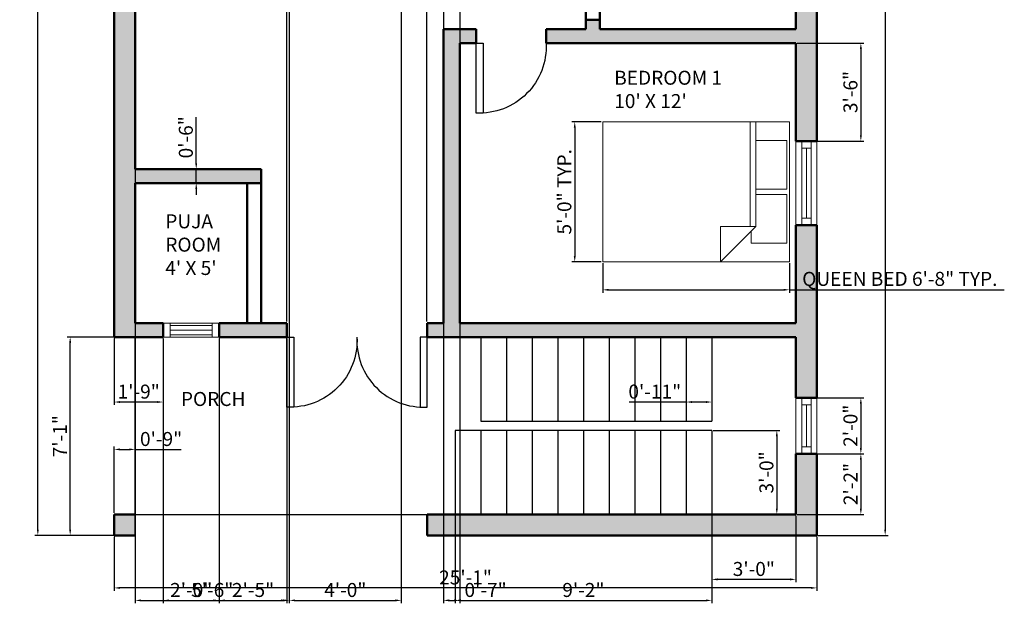
# Model space of a CAD drawing. Units: inches. Extents: x 2247 to 2697, y 1573 to 2133.
# Tile 1 of 4: x 2276 to 2697, y 1573 to 1823. Entities that reach past the tile are written whole.
import ezdxf

# ---------------------------------------------------------------- set-up
doc = ezdxf.new("R2010")
doc.units = ezdxf.units.IN
for name, color, linetype, lineweight in [('A-ANNO-DIMS', 2, 'Continuous', 18), ('A-AREA-IDEN', 7, 'Continuous', 25), ('A-COLS', 7, 'Continuous', 50), ('A-DOOR', 4, 'Continuous', 25), ('A-FLOR', 7, 'Continuous', 25), ('A-FLOR-STRS', 7, 'Continuous', 25), ('A-FURN', 8, 'Continuous', 18), ('A-GLAZ', 4, 'Continuous', 18), ('A-WALL', 7, 'Continuous', 50)]:
    doc.layers.add(name, color=color, linetype=linetype, lineweight=lineweight)
doc.layers.add('A-WALL-PATT', color=67, linetype='Continuous', lineweight=13, true_color=0x727430)
doc.styles.get("Standard").update_dxf_attribs({"font": 'arial.ttf'})
doc.dimstyles.new('ISO-25', dxfattribs={"dimtxt": 6, "dimasz": 2.5, "dimexe": 1.25, "dimexo": 0.625, "dimtad": 1, "dimlunit": 3, "dimtxsty": 'Standard', "dimcen": 2.5, "dimadec": 0, "dimazin": 0, "dimtfac": 1, "dimtmove": 0, "dimatfit": 3, "dimfxl": 1, "dimarcsym": 0})

# ---------------------------------------------------------------- blocks, each defined once
blk = doc.blocks.new('*D2')
at = {"layer": 'A-ANNO-DIMS', "color": 0, "lineweight": -2, "transparency": 16777216}
for p, q in [((2617.72, 2092.36), (2647.6, 2092.36)), ((2646.35, 2089.86), (2646.35, 1604.86)), ((2617.72, 1602.36), (2647.6, 1602.36))]:
    blk.add_line(p, q, dxfattribs=at)
at = {"layer": 'A-ANNO-DIMS', "color": 0, "transparency": 16777216}
for points in [[(2645.94, 2089.86), (2646.77, 2089.86), (2646.35, 2092.36)], [(2645.94, 1604.86), (2646.77, 1604.86), (2646.35, 1602.36)]]:
    blk.add_solid(points, dxfattribs=at)
at = {"layer": 'Defpoints', "color": 0, "transparency": 16777216}
for p in [(2617.09, 2092.36), (2617.09, 1602.36), (2646.35, 1602.36)]:
    blk.add_point(p, dxfattribs=at)
at = {"layer": 'A-ANNO-DIMS', "color": 0, "transparency": 16777216, "insert": (2642.66, 1847.36), "char_height": 6, "attachment_point": 5, "rotation": 90}
blk.add_mtext('40\'-10"', dxfattribs=at)
blk = doc.blocks.new('*D3')
at = {"layer": 'A-ANNO-DIMS', "color": 0, "lineweight": -2, "transparency": 16777216}
for p, q in [((2315.47, 2092.36), (2282.14, 2092.36)), ((2283.39, 1604.86), (2283.39, 2089.86)), ((2315.47, 1602.36), (2282.14, 1602.36))]:
    blk.add_line(p, q, dxfattribs=at)
at = {"layer": 'A-ANNO-DIMS', "color": 0, "transparency": 16777216}
for points in [[(2282.98, 2089.86), (2283.81, 2089.86), (2283.39, 2092.36)], [(2282.98, 1604.86), (2283.81, 1604.86), (2283.39, 1602.36)]]:
    blk.add_solid(points, dxfattribs=at)
at = {"layer": 'Defpoints', "color": 0, "transparency": 16777216}
for p in [(2283.39, 2092.36), (2316.09, 2092.36), (2316.09, 1602.36)]:
    blk.add_point(p, dxfattribs=at)
at = {"layer": 'A-ANNO-DIMS', "color": 0, "transparency": 16777216, "insert": (2279.7, 1847.36), "char_height": 6, "attachment_point": 5, "rotation": 90}
blk.add_mtext('40\'-10"', dxfattribs=at)
blk = doc.blocks.new('*D4')
at = {"layer": 'A-ANNO-DIMS', "color": 0, "lineweight": -2, "transparency": 16777216}
for p, q in [((2316.09, 1601.73), (2316.09, 1578.62)), ((2617.09, 1601.73), (2617.09, 1578.62)), ((2614.59, 1579.87), (2318.59, 1579.87))]:
    blk.add_line(p, q, dxfattribs=at)
at = {"layer": 'A-ANNO-DIMS', "color": 0, "transparency": 16777216}
for points in [[(2318.59, 1580.28), (2318.59, 1579.45), (2316.09, 1579.87)], [(2614.59, 1580.28), (2614.59, 1579.45), (2617.09, 1579.87)]]:
    blk.add_solid(points, dxfattribs=at)
at = {"layer": 'Defpoints', "color": 0, "transparency": 16777216}
for p in [(2316.09, 1602.36), (2617.09, 1602.36), (2316.09, 1579.87)]:
    blk.add_point(p, dxfattribs=at)
at = {"layer": 'A-ANNO-DIMS', "color": 0, "transparency": 16777216, "insert": (2466.59, 1583.56), "char_height": 6, "attachment_point": 5}
blk.add_mtext('25\'-1"', dxfattribs=at)
blk = doc.blocks.new('Bed - Queen')
for p, q in [((0, -80.00003), (0, 0)), ((0, 0), (59.99999, 0)), ((59.99999, 0), (59.99999, -80.00003)), ((7.99999, -1.2), (28.79998, -1.2)), ((7.99999, -14.4), (7.99999, -1.2)), ((28.79998, -1.2), (28.79998, -14.4)), ((31.19999, -1.2), (51.99999, -1.2)), ((31.19999, -14.4), (31.19999, -1.2)), ((51.99999, -1.2), (51.99999, -16.4)), ((0, -14.4), (44.8, -14.4)), ((44.8, -16.8), (0, -16.8)), ((59.99999, -29.6), (44.8, -14.4)), ((44.8, -14.4), (44.8, -29.6)), ((51.99999, -16.4), (46.79936, -16.4)), ((44.8, -29.6), (59.99999, -29.6)), ((59.99999, -80.00003), (0, -80.00003))]:
    blk.add_line(p, q)
blk = doc.blocks.new('DOOR-SWING-30IN')
blk.add_lwpolyline([(0, 0), (3, 0), (3, 30), (0, 30)], close=True)
blk.add_arc((1.5, 1.5), 28.54, 356.9872, 93.0128)
blk = doc.blocks.new('WIN-36IN')
for p, q in [((0, 9), (36, 9)), ((0, 6.5), (36, 6.5)), ((3, 2.5), (3, 6.5)), ((3, 4.5), (33, 4.5)), ((33, 2.5), (33, 6.5)), ((0, 2.5), (36, 2.5)), ((0, 0), (36, 0))]:
    blk.add_line(p, q)
blk = doc.blocks.new('*D15')
at = {"layer": 'A-ANNO-DIMS', "color": 0, "lineweight": -2, "transparency": 16777216}
for p, q in [((2525.38, 1718.97), (2525.38, 1706.35)), ((2605.38, 1718.97), (2605.38, 1706.35)), ((2527.88, 1707.6), (2602.88, 1707.6)), ((2605.38, 1707.6), (2697.39, 1707.6))]:
    blk.add_line(p, q, dxfattribs=at)
at = {"layer": 'A-ANNO-DIMS', "color": 0, "transparency": 16777216}
for points in [[(2527.88, 1708.01), (2527.88, 1707.18), (2525.38, 1707.6)], [(2602.88, 1708.01), (2602.88, 1707.18), (2605.38, 1707.6)]]:
    blk.add_solid(points, dxfattribs=at)
at = {"layer": 'Defpoints', "color": 0, "transparency": 16777216}
for p in [(2525.38, 1719.6), (2605.38, 1719.6), (2605.38, 1707.6)]:
    blk.add_point(p, dxfattribs=at)
at = {"layer": 'A-ANNO-DIMS', "color": 0, "transparency": 16777216, "insert": (2652.63, 1711.51), "char_height": 6, "attachment_point": 5}
blk.add_mtext('QUEEN BED 6\'-8" TYP.', dxfattribs=at)
blk = doc.blocks.new('*D16')
at = {"layer": 'A-ANNO-DIMS', "color": 0, "lineweight": -2, "transparency": 16777216}
for p, q in [((2524.75, 1779.6), (2512.13, 1779.6)), ((2513.38, 1777.1), (2513.38, 1722.1)), ((2524.75, 1719.6), (2512.13, 1719.6))]:
    blk.add_line(p, q, dxfattribs=at)
at = {"layer": 'A-ANNO-DIMS', "color": 0, "transparency": 16777216}
for points in [[(2512.96, 1777.1), (2513.79, 1777.1), (2513.38, 1779.6)], [(2512.96, 1722.1), (2513.79, 1722.1), (2513.38, 1719.6)]]:
    blk.add_solid(points, dxfattribs=at)
at = {"layer": 'Defpoints', "color": 0, "transparency": 16777216}
for p in [(2525.38, 1779.6), (2513.38, 1719.6), (2525.38, 1719.6)]:
    blk.add_point(p, dxfattribs=at)
at = {"layer": 'A-ANNO-DIMS', "color": 0, "transparency": 16777216, "insert": (2509.69, 1749.6), "char_height": 6, "attachment_point": 5, "rotation": 90}
blk.add_mtext('5\'-0" TYP.', dxfattribs=at)
blk = doc.blocks.new('*D26')
at = {"layer": 'A-ANNO-DIMS', "color": 0, "lineweight": -2, "transparency": 16777216}
for p, q in [((2457.09, 2052.73), (2457.09, 1573.26)), ((2464.09, 2052.73), (2464.09, 1573.26)), ((2459.59, 1574.51), (2461.59, 1574.51)), ((2464.09, 1574.51), (2483.79, 1574.51))]:
    blk.add_line(p, q, dxfattribs=at)
at = {"layer": 'A-ANNO-DIMS', "color": 0, "transparency": 16777216}
for points in [[(2459.59, 1574.93), (2459.59, 1574.09), (2457.09, 1574.51)], [(2461.59, 1574.93), (2461.59, 1574.09), (2464.09, 1574.51)]]:
    blk.add_solid(points, dxfattribs=at)
at = {"layer": 'Defpoints', "color": 0, "transparency": 16777216}
for p in [(2457.09, 2053.36), (2464.09, 2053.36), (2464.09, 1574.51)]:
    blk.add_point(p, dxfattribs=at)
at = {"layer": 'A-ANNO-DIMS', "color": 0, "transparency": 16777216, "insert": (2475.19, 1578.2), "char_height": 6, "attachment_point": 5}
blk.add_mtext('0\'-7"', dxfattribs=at)
blk = doc.blocks.new('*D30')
at = {"layer": 'A-ANNO-DIMS', "color": 0, "lineweight": -2, "transparency": 16777216}
for p, q in [((2608.72, 1813.36), (2637.19, 1813.36)), ((2635.94, 1810.86), (2635.94, 1773.86)), ((2608.72, 1771.36), (2637.19, 1771.36))]:
    blk.add_line(p, q, dxfattribs=at)
at = {"layer": 'A-ANNO-DIMS', "color": 0, "transparency": 16777216}
for points in [[(2635.53, 1810.86), (2636.36, 1810.86), (2635.94, 1813.36)], [(2635.53, 1773.86), (2636.36, 1773.86), (2635.94, 1771.36)]]:
    blk.add_solid(points, dxfattribs=at)
at = {"layer": 'Defpoints', "color": 0, "transparency": 16777216}
for p in [(2608.09, 1813.36), (2608.09, 1771.36), (2635.94, 1771.36)]:
    blk.add_point(p, dxfattribs=at)
at = {"layer": 'A-ANNO-DIMS', "color": 0, "transparency": 16777216, "insert": (2632.25, 1792.36), "char_height": 6, "attachment_point": 5, "rotation": 90}
blk.add_mtext('3\'-6"', dxfattribs=at)
blk = doc.blocks.new('*D31')
at = {"layer": 'A-ANNO-DIMS', "color": 0, "lineweight": -2, "transparency": 16777216}
for p, q in [((2608.72, 1637.36), (2637.19, 1637.36)), ((2635.94, 1634.86), (2635.94, 1613.86)), ((2608.72, 1611.36), (2637.19, 1611.36))]:
    blk.add_line(p, q, dxfattribs=at)
at = {"layer": 'A-ANNO-DIMS', "color": 0, "transparency": 16777216}
for points in [[(2635.53, 1634.86), (2636.36, 1634.86), (2635.94, 1637.36)], [(2635.53, 1613.86), (2636.36, 1613.86), (2635.94, 1611.36)]]:
    blk.add_solid(points, dxfattribs=at)
at = {"layer": 'Defpoints', "color": 0, "transparency": 16777216}
for p in [(2608.09, 1637.36), (2608.09, 1611.36), (2635.94, 1611.36)]:
    blk.add_point(p, dxfattribs=at)
at = {"layer": 'A-ANNO-DIMS', "color": 0, "transparency": 16777216, "insert": (2632.31, 1624.36), "char_height": 6, "attachment_point": 5, "rotation": 90}
blk.add_mtext('2\'-2"', dxfattribs=at)
blk = doc.blocks.new('*D32')
at = {"layer": 'A-ANNO-DIMS', "color": 0, "lineweight": -2, "transparency": 16777216}
for p, q in [((2608.72, 1661.36), (2637.19, 1661.36)), ((2635.94, 1658.86), (2635.94, 1639.86)), ((2608.72, 1637.36), (2637.19, 1637.36))]:
    blk.add_line(p, q, dxfattribs=at)
at = {"layer": 'A-ANNO-DIMS', "color": 0, "transparency": 16777216}
for points in [[(2635.53, 1658.86), (2636.36, 1658.86), (2635.94, 1661.36)], [(2635.53, 1639.86), (2636.36, 1639.86), (2635.94, 1637.36)]]:
    blk.add_solid(points, dxfattribs=at)
at = {"layer": 'Defpoints', "color": 0, "transparency": 16777216}
for p in [(2608.09, 1661.36), (2608.09, 1637.36), (2635.94, 1637.36)]:
    blk.add_point(p, dxfattribs=at)
at = {"layer": 'A-ANNO-DIMS', "color": 0, "transparency": 16777216, "insert": (2632.26, 1649.36), "char_height": 6, "attachment_point": 5, "rotation": 90}
blk.add_mtext('2\'-0"', dxfattribs=at)
blk = doc.blocks.new('*D33')
at = {"layer": 'A-ANNO-DIMS', "color": 0, "lineweight": -2, "transparency": 16777216}
for p, q in [((2324.47, 1687.36), (2295.99, 1687.36)), ((2297.24, 1604.86), (2297.24, 1684.86)), ((2324.47, 1602.36), (2295.99, 1602.36))]:
    blk.add_line(p, q, dxfattribs=at)
at = {"layer": 'A-ANNO-DIMS', "color": 0, "transparency": 16777216}
for points in [[(2296.83, 1684.86), (2297.66, 1684.86), (2297.24, 1687.36)], [(2296.83, 1604.86), (2297.66, 1604.86), (2297.24, 1602.36)]]:
    blk.add_solid(points, dxfattribs=at)
at = {"layer": 'Defpoints', "color": 0, "transparency": 16777216}
for p in [(2297.24, 1687.36), (2325.09, 1687.36), (2325.09, 1602.36)]:
    blk.add_point(p, dxfattribs=at)
at = {"layer": 'A-ANNO-DIMS', "color": 0, "transparency": 16777216, "insert": (2293.61, 1644.86), "char_height": 6, "attachment_point": 5, "rotation": 90}
blk.add_mtext('7\'-1"', dxfattribs=at)
blk = doc.blocks.new('*D34')
at = {"layer": 'A-ANNO-DIMS', "color": 0, "lineweight": -2, "transparency": 16777216}
for p, q in [((2316.09, 1611.98), (2316.09, 1640.46)), ((2318.59, 1639.21), (2322.59, 1639.21)), ((2325.09, 1611.98), (2325.09, 1640.46)), ((2325.09, 1639.21), (2344.79, 1639.21))]:
    blk.add_line(p, q, dxfattribs=at)
at = {"layer": 'A-ANNO-DIMS', "color": 0, "transparency": 16777216}
for points in [[(2318.59, 1639.63), (2318.59, 1638.79), (2316.09, 1639.21)], [(2322.59, 1639.63), (2322.59, 1638.79), (2325.09, 1639.21)]]:
    blk.add_solid(points, dxfattribs=at)
at = {"layer": 'Defpoints', "color": 0, "transparency": 16777216}
for p in [(2325.09, 1639.21), (2316.09, 1611.36), (2325.09, 1611.36)]:
    blk.add_point(p, dxfattribs=at)
at = {"layer": 'A-ANNO-DIMS', "color": 0, "transparency": 16777216, "insert": (2336.19, 1642.9), "char_height": 6, "attachment_point": 5}
blk.add_mtext('0\'-9"', dxfattribs=at)
blk = doc.blocks.new('*D35')
at = {"layer": 'A-ANNO-DIMS', "color": 0, "lineweight": -2, "transparency": 16777216}
for p, q in [((2316.09, 1686.73), (2316.09, 1658.26)), ((2337.09, 1686.73), (2337.09, 1658.26)), ((2334.59, 1659.51), (2318.59, 1659.51))]:
    blk.add_line(p, q, dxfattribs=at)
at = {"layer": 'A-ANNO-DIMS', "color": 0, "transparency": 16777216}
for points in [[(2318.59, 1659.93), (2318.59, 1659.09), (2316.09, 1659.51)], [(2334.59, 1659.93), (2334.59, 1659.09), (2337.09, 1659.51)]]:
    blk.add_solid(points, dxfattribs=at)
at = {"layer": 'Defpoints', "color": 0, "transparency": 16777216}
for p in [(2316.09, 1687.36), (2337.09, 1687.36), (2316.09, 1659.51)]:
    blk.add_point(p, dxfattribs=at)
at = {"layer": 'A-ANNO-DIMS', "color": 0, "transparency": 16777216, "insert": (2326.59, 1663.2), "char_height": 6, "attachment_point": 5}
blk.add_mtext('1\'-9"', dxfattribs=at)
blk = doc.blocks.new('*D36')
at = {"layer": 'A-ANNO-DIMS', "color": 0, "lineweight": -2, "transparency": 16777216}
for p, q in [((2337.09, 1686.73), (2337.09, 1573.26)), ((2361.09, 1686.73), (2361.09, 1573.26)), ((2339.59, 1574.51), (2358.59, 1574.51))]:
    blk.add_line(p, q, dxfattribs=at)
at = {"layer": 'A-ANNO-DIMS', "color": 0, "transparency": 16777216}
for points in [[(2339.59, 1574.93), (2339.59, 1574.09), (2337.09, 1574.51)], [(2358.59, 1574.93), (2358.59, 1574.09), (2361.09, 1574.51)]]:
    blk.add_solid(points, dxfattribs=at)
at = {"layer": 'Defpoints', "color": 0, "transparency": 16777216}
for p in [(2337.09, 1687.36), (2361.09, 1687.36), (2361.09, 1574.51)]:
    blk.add_point(p, dxfattribs=at)
at = {"layer": 'A-ANNO-DIMS', "color": 0, "transparency": 16777216, "insert": (2349.09, 1578.2), "char_height": 6, "attachment_point": 5}
blk.add_mtext('2\'-0"', dxfattribs=at)
blk = doc.blocks.new('*D37')
at = {"layer": 'A-ANNO-DIMS', "color": 0, "lineweight": -2, "transparency": 16777216}
for p, q in [((2361.09, 1686.73), (2361.09, 1573.26)), ((2390.09, 1686.73), (2390.09, 1573.26)), ((2363.59, 1574.51), (2387.59, 1574.51))]:
    blk.add_line(p, q, dxfattribs=at)
at = {"layer": 'A-ANNO-DIMS', "color": 0, "transparency": 16777216}
for points in [[(2363.59, 1574.93), (2363.59, 1574.09), (2361.09, 1574.51)], [(2387.59, 1574.93), (2387.59, 1574.09), (2390.09, 1574.51)]]:
    blk.add_solid(points, dxfattribs=at)
at = {"layer": 'Defpoints', "color": 0, "transparency": 16777216}
for p in [(2361.09, 1687.36), (2390.09, 1687.36), (2390.09, 1574.51)]:
    blk.add_point(p, dxfattribs=at)
at = {"layer": 'A-ANNO-DIMS', "color": 0, "transparency": 16777216, "insert": (2375.59, 1578.2), "char_height": 6, "attachment_point": 5}
blk.add_mtext('2\'-5"', dxfattribs=at)
blk = doc.blocks.new('*D38')
at = {"layer": 'A-ANNO-DIMS', "color": 0, "lineweight": -2, "transparency": 16777216}
for p, q in [((2390.09, 1693.98), (2390.09, 2121.46)), ((2392.59, 2120.21), (2447.59, 2120.21)), ((2450.09, 1693.98), (2450.09, 2121.46))]:
    blk.add_line(p, q, dxfattribs=at)
at = {"layer": 'A-ANNO-DIMS', "color": 0, "transparency": 16777216}
for points in [[(2392.59, 2120.63), (2392.59, 2119.79), (2390.09, 2120.21)], [(2447.59, 2120.63), (2447.59, 2119.79), (2450.09, 2120.21)]]:
    blk.add_solid(points, dxfattribs=at)
at = {"layer": 'Defpoints', "color": 0, "transparency": 16777216}
for p in [(2450.09, 2120.21), (2390.09, 1693.36), (2450.09, 1693.36)]:
    blk.add_point(p, dxfattribs=at)
at = {"layer": 'A-ANNO-DIMS', "color": 0, "transparency": 16777216, "insert": (2420.09, 2123.9), "char_height": 6, "attachment_point": 5}
blk.add_mtext('5\'-0"', dxfattribs=at)
blk = doc.blocks.new('*D39')
at = {"layer": 'A-ANNO-DIMS', "color": 0, "lineweight": -2, "transparency": 16777216}
for p, q in [((2325.09, 1992.73), (2325.09, 1573.26)), ((2391.09, 1992.73), (2391.09, 1573.26)), ((2327.59, 1574.51), (2388.59, 1574.51))]:
    blk.add_line(p, q, dxfattribs=at)
at = {"layer": 'A-ANNO-DIMS', "color": 0, "transparency": 16777216}
for points in [[(2327.59, 1574.93), (2327.59, 1574.09), (2325.09, 1574.51)], [(2388.59, 1574.93), (2388.59, 1574.09), (2391.09, 1574.51)]]:
    blk.add_solid(points, dxfattribs=at)
at = {"layer": 'Defpoints', "color": 0, "transparency": 16777216}
for p in [(2325.09, 1993.36), (2391.09, 1993.36), (2391.09, 1574.51)]:
    blk.add_point(p, dxfattribs=at)
at = {"layer": 'A-ANNO-DIMS', "color": 0, "transparency": 16777216, "insert": (2358.09, 1578.2), "char_height": 6, "attachment_point": 5}
blk.add_mtext('5\'-6"', dxfattribs=at)
blk = doc.blocks.new('*D40')
at = {"layer": 'A-ANNO-DIMS', "color": 0, "lineweight": -2, "transparency": 16777216}
for p, q in [((2391.09, 1992.73), (2391.09, 1573.26)), ((2439.09, 1992.73), (2439.09, 1573.26)), ((2393.59, 1574.51), (2436.59, 1574.51))]:
    blk.add_line(p, q, dxfattribs=at)
at = {"layer": 'A-ANNO-DIMS', "color": 0, "transparency": 16777216}
for points in [[(2393.59, 1574.93), (2393.59, 1574.09), (2391.09, 1574.51)], [(2436.59, 1574.93), (2436.59, 1574.09), (2439.09, 1574.51)]]:
    blk.add_solid(points, dxfattribs=at)
at = {"layer": 'Defpoints', "color": 0, "transparency": 16777216}
for p in [(2391.09, 1993.36), (2439.09, 1993.36), (2439.09, 1574.51)]:
    blk.add_point(p, dxfattribs=at)
at = {"layer": 'A-ANNO-DIMS', "color": 0, "transparency": 16777216, "insert": (2415.09, 1578.2), "char_height": 6, "attachment_point": 5}
blk.add_mtext('4\'-0"', dxfattribs=at)
blk = doc.blocks.new('*D41')
at = {"layer": 'A-ANNO-DIMS', "color": 0, "lineweight": -2, "transparency": 16777216}
for p, q in [((2351.24, 1761.86), (2351.24, 1781.56)), ((2378.47, 1759.36), (2349.99, 1759.36)), ((2351.24, 1753.36), (2351.24, 1759.36)), ((2378.47, 1753.36), (2349.99, 1753.36)), ((2351.24, 1750.86), (2351.24, 1748.36))]:
    blk.add_line(p, q, dxfattribs=at)
at = {"layer": 'A-ANNO-DIMS', "color": 0, "transparency": 16777216}
for points in [[(2350.83, 1761.86), (2351.66, 1761.86), (2351.24, 1759.36)], [(2350.83, 1750.86), (2351.66, 1750.86), (2351.24, 1753.36)]]:
    blk.add_solid(points, dxfattribs=at)
at = {"layer": 'Defpoints', "color": 0, "transparency": 16777216}
for p in [(2351.24, 1759.36), (2379.09, 1759.36), (2379.09, 1753.36)]:
    blk.add_point(p, dxfattribs=at)
at = {"layer": 'A-ANNO-DIMS', "color": 0, "transparency": 16777216, "insert": (2347.56, 1772.96), "char_height": 6, "attachment_point": 5, "rotation": 90}
blk.add_mtext('0\'-6"', dxfattribs=at)
blk = doc.blocks.new('*D45')
at = {"layer": 'A-ANNO-DIMS', "color": 0, "lineweight": -2, "transparency": 16777216}
for p, q in [((2462.09, 1610.73), (2462.09, 1573.26)), ((2572.09, 1610.73), (2572.09, 1573.26)), ((2464.59, 1574.51), (2569.59, 1574.51))]:
    blk.add_line(p, q, dxfattribs=at)
at = {"layer": 'A-ANNO-DIMS', "color": 0, "transparency": 16777216}
for points in [[(2464.59, 1574.93), (2464.59, 1574.09), (2462.09, 1574.51)], [(2569.59, 1574.93), (2569.59, 1574.09), (2572.09, 1574.51)]]:
    blk.add_solid(points, dxfattribs=at)
at = {"layer": 'Defpoints', "color": 0, "transparency": 16777216}
for p in [(2462.09, 1611.36), (2572.09, 1611.36), (2572.09, 1574.51)]:
    blk.add_point(p, dxfattribs=at)
at = {"layer": 'A-ANNO-DIMS', "color": 0, "transparency": 16777216, "insert": (2517.09, 1578.2), "char_height": 6, "attachment_point": 5}
blk.add_mtext('9\'-2"', dxfattribs=at)
blk = doc.blocks.new('*D46')
at = {"layer": 'A-ANNO-DIMS', "color": 0, "lineweight": -2, "transparency": 16777216}
for p, q in [((2572.09, 1610.73), (2572.09, 1582.26)), ((2608.09, 1610.73), (2608.09, 1582.26)), ((2605.59, 1583.51), (2574.59, 1583.51))]:
    blk.add_line(p, q, dxfattribs=at)
at = {"layer": 'A-ANNO-DIMS', "color": 0, "transparency": 16777216}
for points in [[(2574.59, 1583.93), (2574.59, 1583.09), (2572.09, 1583.51)], [(2605.59, 1583.93), (2605.59, 1583.09), (2608.09, 1583.51)]]:
    blk.add_solid(points, dxfattribs=at)
at = {"layer": 'Defpoints', "color": 0, "transparency": 16777216}
for p in [(2572.09, 1611.36), (2608.09, 1611.36), (2572.09, 1583.51)]:
    blk.add_point(p, dxfattribs=at)
at = {"layer": 'A-ANNO-DIMS', "color": 0, "transparency": 16777216, "insert": (2590.09, 1587.2), "char_height": 6, "attachment_point": 5}
blk.add_mtext('3\'-0"', dxfattribs=at)
blk = doc.blocks.new('*D47')
at = {"layer": 'A-ANNO-DIMS', "color": 0, "lineweight": -2, "transparency": 16777216}
for p, q in [((2572.72, 1647.36), (2601.19, 1647.36)), ((2599.94, 1644.86), (2599.94, 1613.86)), ((2572.72, 1611.36), (2601.19, 1611.36))]:
    blk.add_line(p, q, dxfattribs=at)
at = {"layer": 'A-ANNO-DIMS', "color": 0, "transparency": 16777216}
for points in [[(2599.53, 1644.86), (2600.36, 1644.86), (2599.94, 1647.36)], [(2599.53, 1613.86), (2600.36, 1613.86), (2599.94, 1611.36)]]:
    blk.add_solid(points, dxfattribs=at)
at = {"layer": 'Defpoints', "color": 0, "transparency": 16777216}
for p in [(2572.09, 1647.36), (2572.09, 1611.36), (2599.94, 1611.36)]:
    blk.add_point(p, dxfattribs=at)
at = {"layer": 'A-ANNO-DIMS', "color": 0, "transparency": 16777216, "insert": (2596.25, 1629.36), "char_height": 6, "attachment_point": 5, "rotation": 90}
blk.add_mtext('3\'-0"', dxfattribs=at)
blk = doc.blocks.new('*D48')
at = {"layer": 'A-ANNO-DIMS', "color": 0, "lineweight": -2, "transparency": 16777216}
for p, q in [((2561.09, 1686.73), (2561.09, 1658.26)), ((2572.09, 1686.73), (2572.09, 1658.26)), ((2561.09, 1659.51), (2536.73, 1659.51)), ((2569.59, 1659.51), (2563.59, 1659.51))]:
    blk.add_line(p, q, dxfattribs=at)
at = {"layer": 'A-ANNO-DIMS', "color": 0, "transparency": 16777216}
for points in [[(2563.59, 1659.93), (2563.59, 1659.09), (2561.09, 1659.51)], [(2569.59, 1659.93), (2569.59, 1659.09), (2572.09, 1659.51)]]:
    blk.add_solid(points, dxfattribs=at)
at = {"layer": 'Defpoints', "color": 0, "transparency": 16777216}
for p in [(2561.09, 1687.36), (2572.09, 1687.36), (2561.09, 1659.51)]:
    blk.add_point(p, dxfattribs=at)
at = {"layer": 'A-ANNO-DIMS', "color": 0, "transparency": 16777216, "insert": (2547.66, 1663.2), "char_height": 6, "attachment_point": 5}
blk.add_mtext('0\'-11"', dxfattribs=at)

msp = doc.modelspace()

# ---------------------------------------------------------------- hatches: boundary and pattern name
at = {"layer": 'A-WALL-PATT'}
h = msp.add_hatch(color=256, dxfattribs=at)
h.dxf.hatch_style = 1
h.paths.add_polyline_path([(2325.094, 1993.36), (2391.094, 1993.36), (2391.094, 1999.36), (2325.094, 1999.36), (2325.094, 2083.36), (2373.094, 2083.36), (2373.094, 2092.36), (2316.094, 2092.36), (2316.094, 1687.36), (2337.094, 1687.36), (2337.094, 1693.36), (2325.094, 1693.36), (2325.094, 1753.36), (2379.094, 1753.36), (2379.094, 1759.36), (2325.094, 1759.36)])
h = msp.add_hatch(color=256, dxfattribs=at)
h.dxf.hatch_style = 1
h.paths.add_polyline_path([(2617.094, 1837.36), (2608.094, 1837.36), (2608.094, 1819.36), (2524.094, 1819.36), (2524.094, 1823.36), (2518.094, 1823.36), (2518.094, 1819.36), (2501.094, 1819.36), (2501.094, 1813.36), (2608.094, 1813.36), (2608.094, 1771.36), (2617.094, 1771.36)])
h = msp.add_hatch(color=256, dxfattribs=at)
h.dxf.hatch_style = 1
h.paths.add_polyline_path([(2617.094, 1735.36), (2608.094, 1735.36), (2608.094, 1693.36), (2464.094, 1693.36), (2464.094, 1813.36), (2471.094, 1813.36), (2471.094, 1819.36), (2457.094, 1819.36), (2457.094, 1693.36), (2450.094, 1693.36), (2450.094, 1687.36), (2608.094, 1687.36), (2608.094, 1661.36), (2617.094, 1661.36)])
h = msp.add_hatch(color=256, dxfattribs=at)
h.dxf.hatch_style = 1
h.paths.add_polyline_path([(2390.094, 1693.36), (2379.094, 1693.36), (2361.094, 1693.36), (2361.094, 1687.36), (2390.094, 1687.36)])
h = msp.add_hatch(color=256, dxfattribs=at)
h.dxf.hatch_style = 1
h.paths.add_polyline_path([(2617.094, 1637.36), (2608.094, 1637.36), (2608.094, 1611.36), (2450.094, 1611.36), (2450.094, 1602.36), (2617.094, 1602.36)])
h = msp.add_hatch(color=256, dxfattribs=at)
h.dxf.hatch_style = 1
h.paths.add_polyline_path([(2325.094, 1611.36), (2316.094, 1611.36), (2316.094, 1602.36), (2325.094, 1602.36)])

# ---------------------------------------------------------------- linework, layer by layer
at = {"layer": 'A-COLS'}
msp.add_line((2325.094, 1611.36), (2316.094, 1611.36), dxfattribs=at)
msp.add_lwpolyline([(2325.094, 1602.36), (2316.094, 1602.36), (2316.094, 1611.36)], dxfattribs=at)
at = {"layer": 'A-FLOR'}
for p, q in [((2325.094, 1602.36), (2325.094, 1687.36)), ((2325.094, 1611.36), (2450.094, 1611.36))]:
    msp.add_line(p, q, dxfattribs=at)
at = {"layer": 'A-FLOR-STRS'}
for p, q in [((2473.094, 1687.36), (2473.094, 1651.36)), ((2484.094, 1687.36), (2484.094, 1651.36)), ((2495.094, 1687.36), (2495.094, 1651.36)), ((2506.094, 1687.36), (2506.094, 1651.36)), ((2517.094, 1687.36), (2517.094, 1651.36)), ((2528.094, 1687.36), (2528.094, 1651.36)), ((2539.094, 1687.36), (2539.094, 1651.36)), ((2550.094, 1687.36), (2550.094, 1651.36)), ((2561.094, 1687.36), (2561.094, 1651.36)), ((2572.094, 1687.36), (2572.094, 1651.36)), ((2473.094, 1651.36), (2572.094, 1651.36)), ((2572.094, 1647.36), (2462.094, 1647.36)), ((2462.094, 1647.36), (2462.094, 1611.36)), ((2473.094, 1647.36), (2473.094, 1611.36)), ((2484.094, 1647.36), (2484.094, 1611.36)), ((2495.094, 1647.36), (2495.094, 1611.36)), ((2506.094, 1647.36), (2506.094, 1611.36)), ((2517.094, 1647.36), (2517.094, 1611.36)), ((2528.094, 1647.36), (2528.094, 1611.36)), ((2539.094, 1647.36), (2539.094, 1611.36)), ((2550.094, 1647.36), (2550.094, 1611.36)), ((2561.094, 1647.36), (2561.094, 1611.36)), ((2572.094, 1647.36), (2572.094, 1611.36))]:
    msp.add_line(p, q, dxfattribs=at)
at = {"layer": 'A-GLAZ'}
for p, q in [((2337.094, 1693.36), (2361.094, 1693.36)), ((2340.094, 1693.36), (2340.094, 1687.36)), ((2340.094, 1692.36), (2358.094, 1692.36)), ((2358.094, 1693.36), (2358.094, 1687.36)), ((2337.094, 1687.36), (2361.094, 1687.36)), ((2340.094, 1690.36), (2358.094, 1690.36)), ((2340.094, 1688.36), (2358.094, 1688.36)), ((2608.094, 1661.36), (2608.094, 1637.36)), ((2610.594, 1637.36), (2610.594, 1661.36)), ((2610.594, 1658.36), (2614.594, 1658.36)), ((2612.594, 1640.36), (2612.594, 1658.36)), ((2614.594, 1637.36), (2614.594, 1661.36)), ((2617.094, 1637.36), (2617.094, 1661.36)), ((2610.594, 1640.36), (2614.594, 1640.36))]:
    msp.add_line(p, q, dxfattribs=at)
at = {"layer": 'A-WALL'}
for p, q in [((2325.094, 1759.36), (2325.094, 1993.36)), ((2518.094, 1823.36), (2518.094, 1863.36)), ((2524.094, 1823.36), (2524.094, 1863.36)), ((2608.094, 1837.36), (2608.094, 1819.36)), ((2518.094, 1823.36), (2524.094, 1823.36)), ((2518.094, 1823.36), (2518.094, 1819.36)), ((2524.094, 1823.36), (2524.094, 1819.36)), ((2457.094, 1819.36), (2471.094, 1819.36)), ((2457.094, 1693.36), (2457.094, 1819.36)), ((2471.094, 1813.36), (2471.094, 1819.36)), ((2501.094, 1813.36), (2501.094, 1819.36)), ((2501.094, 1819.36), (2518.094, 1819.36)), ((2524.094, 1819.36), (2608.094, 1819.36)), ((2464.094, 1813.36), (2471.094, 1813.36)), ((2464.094, 1813.36), (2464.094, 1693.36)), ((2501.094, 1813.36), (2608.094, 1813.36)), ((2608.094, 1813.36), (2608.094, 1771.36)), ((2608.094, 1771.36), (2617.094, 1771.36)), ((2325.094, 1759.36), (2379.094, 1759.36)), ((2379.094, 1693.36), (2379.094, 1759.36)), ((2325.094, 1753.36), (2379.094, 1753.36)), ((2325.094, 1693.36), (2325.094, 1753.36)), ((2373.094, 1693.36), (2373.094, 1753.36)), ((2608.094, 1735.36), (2617.094, 1735.36)), ((2608.094, 1735.36), (2608.094, 1693.36)), ((2325.094, 1693.36), (2337.094, 1693.36)), ((2325.094, 1693.36), (2337.094, 1693.36)), ((2337.094, 1693.36), (2337.094, 1687.36)), ((2361.094, 1693.36), (2361.094, 1687.36)), ((2361.094, 1693.36), (2379.094, 1693.36)), ((2379.094, 1693.36), (2390.094, 1693.36)), ((2390.094, 1693.36), (2390.094, 1687.36)), ((2450.094, 1693.36), (2450.094, 1687.36)), ((2450.094, 1693.36), (2457.094, 1693.36)), ((2464.094, 1693.36), (2608.094, 1693.36)), ((2316.094, 1687.36), (2337.094, 1687.36)), ((2361.094, 1687.36), (2390.094, 1687.36)), ((2450.094, 1687.36), (2608.094, 1687.36)), ((2608.094, 1687.36), (2608.094, 1661.36)), ((2608.094, 1661.36), (2617.094, 1661.36)), ((2608.094, 1637.36), (2617.094, 1637.36)), ((2608.094, 1637.36), (2608.094, 1611.36)), ((2608.094, 1611.36), (2450.094, 1611.36)), ((2450.094, 1611.36), (2450.094, 1602.36))]:
    msp.add_line(p, q, dxfattribs=at)
for points in [[(2316.094, 1687.36), (2316.094, 2092.36), (2373.094, 2092.36)], [(2617.094, 1837.36), (2617.094, 1771.36)], [(2617.094, 1735.36), (2617.094, 1661.36)], [(2617.094, 1637.36), (2617.094, 1602.36), (2450.094, 1602.36)]]:
    msp.add_lwpolyline(points, dxfattribs=at)

# ---------------------------------------------------------------- block references
at = {"layer": 'A-DOOR', "extrusion": (0, 0, -1), "zscale": -1, "rotation": 180}
for p in [(-2471.094, 1813.359), (-2390.094, 1687.359)]:
    msp.add_blockref('DOOR-SWING-30IN', p, dxfattribs=at)
at = {"layer": 'A-DOOR', "rotation": 180}
msp.add_blockref('DOOR-SWING-30IN', (2450.095, 1687.359), dxfattribs=at)
at = {"layer": 'A-FURN', "rotation": 270}
msp.add_blockref('Bed - Queen', (2605.377, 1779.598), dxfattribs=at)
at = {"layer": 'A-GLAZ', "rotation": 270.0000000000046}
msp.add_blockref('WIN-36IN', (2608.095, 1771.36), dxfattribs=at)

# ---------------------------------------------------------------- texts
at = {"layer": 'A-AREA-IDEN', "char_height": 6, "attachment_point": 1}
for s, width, insert in [("{\\fArial|b1|i0|c0|p34;BEDROOM 1 \\P10' X 12' }", 56.09422, (2530.288, 1801.481)), ("{\\fArial|b1|i0|c0|p34;PUJA ROOM\\P4' X 5'}", 28.99459, (2337.975, 1739.957)), ('{\\fArial|b1|i0|c0|p34;PORCH }', 85.16828, (2344.675, 1663.817))]:
    msp.add_mtext_dynamic_manual_height_columns(s, width=width, gutter_width=12.5, heights=[0], dxfattribs=dict(at, insert=insert))

# ---------------------------------------------------------------- dimensions: what is measured, and where the dimension line sits
at = {"layer": 'A-ANNO-DIMS'}
for base, p1, p2, override, picture, middle in [((2450.094, 2120.21), (2390.094, 1693.36), (2450.094, 1693.36), {"dimdec": 1, "dimlfac": 1, "dimrnd": 0, "dimzin": 1, "dimdsep": 46, "dimlunit": 4, "dimfrac": 2}, '*D38', (2420.094, 2123.898)), ((2464.094, 1574.51), (2457.094, 2053.36), (2464.094, 2053.36), {"dimdec": 1, "dimlfac": 1, "dimrnd": 0, "dimzin": 1, "dimdsep": 46, "dimlunit": 4, "dimfrac": 2}, '*D26', (2475.194, 1578.198)), ((2391.094, 1574.51), (2325.094, 1993.36), (2391.094, 1993.36), {"dimdec": 1, "dimlfac": 1, "dimrnd": 0, "dimzin": 1, "dimdsep": 46, "dimlunit": 4, "dimfrac": 2}, '*D39', (2358.094, 1578.198)), ((2439.094, 1574.51), (2391.094, 1993.36), (2439.094, 1993.36), {"dimdec": 1, "dimlfac": 1, "dimrnd": 0, "dimzin": 1, "dimdsep": 46, "dimlunit": 4, "dimfrac": 2}, '*D40', (2415.094, 1578.198)), ((2361.094, 1574.51), (2337.094, 1687.36), (2361.094, 1687.36), {"dimdec": 1, "dimlfac": 1, "dimrnd": 0, "dimzin": 1, "dimdsep": 46, "dimlunit": 4, "dimfrac": 2}, '*D36', (2349.094, 1578.198)), ((2390.094, 1574.51), (2361.094, 1687.36), (2390.094, 1687.36), {"dimdec": 1, "dimlfac": 1, "dimrnd": 0, "dimzin": 1, "dimdsep": 46, "dimlunit": 4, "dimfrac": 2}, '*D37', (2375.594, 1578.198)), ((2325.094, 1639.21), (2316.094, 1611.36), (2325.094, 1611.36), {"dimdec": 1, "dimlfac": 1, "dimrnd": 0, "dimzin": 1, "dimdsep": 46, "dimlunit": 4, "dimfrac": 2}, '*D34', (2336.194, 1642.898)), ((2572.094, 1574.51), (2462.094, 1611.36), (2572.094, 1611.36), {"dimdec": 1, "dimlfac": 1, "dimrnd": 0, "dimzin": 1, "dimdsep": 46, "dimlunit": 4, "dimfrac": 2}, '*D45', (2517.094, 1578.198)), ((2316.094, 1579.868), (2617.094, 1602.36), (2316.094, 1602.36), {"dimclrd": 0, "dimclre": 0, "dimclrt": 0}, '*D4', (2466.594, 1583.556))]:
    dim = msp.add_linear_dim(base=base, p1=p1, p2=p2, dimstyle='ISO-25', override=override, dxfattribs=at)
    dim.commit()
    dim.dimension.update_dxf_attribs({"geometry": picture, "text_midpoint": middle})
for base, p1, p2, angle, override, picture, middle in [((2283.393, 2092.36), (2316.094, 1602.36), (2316.094, 2092.36), 90, {"dimclrd": 0, "dimclre": 0, "dimclrt": 0}, '*D3', (2279.704, 1847.36)), ((2646.352, 1602.36), (2617.094, 2092.36), (2617.094, 1602.36), 90, {"dimclrd": 0, "dimclre": 0, "dimclrt": 0}, '*D2', (2642.664, 1847.36)), ((2635.944, 1771.36), (2608.094, 1813.36), (2608.094, 1771.36), 270, {"dimdec": 1, "dimlfac": 1, "dimrnd": 0, "dimzin": 1, "dimdsep": 46, "dimlunit": 4, "dimfrac": 2}, '*D30', (2632.254, 1792.36)), ((2351.244, 1759.36), (2379.094, 1753.36), (2379.094, 1759.36), 90, {"dimdec": 1, "dimlfac": 1, "dimrnd": 0, "dimzin": 1, "dimdsep": 46, "dimlunit": 4, "dimfrac": 2}, '*D41', (2347.556, 1772.959)), ((2297.244, 1687.36), (2325.094, 1602.36), (2325.094, 1687.36), 90, {"dimdec": 1, "dimlfac": 1, "dimrnd": 0, "dimzin": 1, "dimdsep": 46, "dimlunit": 4, "dimfrac": 2}, '*D33', (2293.607, 1644.86)), ((2316.094, 1659.51), (2337.094, 1687.36), (2316.094, 1687.36), 180, {"dimdec": 1, "dimlfac": 1, "dimrnd": 0, "dimzin": 1, "dimdsep": 46, "dimlunit": 4, "dimfrac": 2}, '*D35', (2326.594, 1663.198)), ((2561.094, 1659.51), (2572.094, 1687.36), (2561.094, 1687.36), 180, {"dimdec": 1, "dimlfac": 1, "dimrnd": 0, "dimzin": 1, "dimdsep": 46, "dimlunit": 4, "dimfrac": 2}, '*D48', (2547.664, 1663.198)), ((2635.944, 1637.36), (2608.094, 1661.36), (2608.094, 1637.36), 270, {"dimdec": 1, "dimlfac": 1, "dimrnd": 0, "dimzin": 1, "dimdsep": 46, "dimlunit": 4, "dimfrac": 2}, '*D32', (2632.256, 1649.36)), ((2599.944, 1611.36), (2572.094, 1647.36), (2572.094, 1611.36), 270, {"dimdec": 1, "dimlfac": 1, "dimrnd": 0, "dimzin": 1, "dimdsep": 46, "dimlunit": 4, "dimfrac": 2}, '*D47', (2596.254, 1629.36)), ((2635.944, 1611.36), (2608.094, 1637.36), (2608.094, 1611.36), 270, {"dimdec": 1, "dimlfac": 1, "dimrnd": 0, "dimzin": 1, "dimdsep": 46, "dimlunit": 4, "dimfrac": 2}, '*D31', (2632.307, 1624.36)), ((2572.094, 1583.51), (2608.094, 1611.36), (2572.094, 1611.36), 180, {"dimdec": 1, "dimlfac": 1, "dimrnd": 0, "dimzin": 1, "dimdsep": 46, "dimlunit": 4, "dimfrac": 2}, '*D46', (2590.094, 1587.2))]:
    dim = msp.add_linear_dim(base=base, p1=p1, p2=p2, angle=angle, dimstyle='ISO-25', override=override, dxfattribs=at)
    dim.commit()
    dim.dimension.update_dxf_attribs({"geometry": picture, "text_midpoint": middle})
dim = msp.add_linear_dim(base=(2513.377, 1719.598), p1=(2525.377, 1779.598), p2=(2525.377, 1719.598), angle=270, text='<> TYP.', dimstyle='ISO-25', override={"dimdec": 1, "dimlfac": 1, "dimrnd": 0, "dimzin": 1, "dimdsep": 46, "dimlunit": 4, "dimfrac": 2}, dxfattribs=at)
dim.commit()
dim.dimension.update_dxf_attribs({"geometry": '*D16', "text_midpoint": (2509.689, 1749.598)})
dim = msp.add_linear_dim(base=(2605.377, 1707.598), p1=(2525.377, 1719.598), p2=(2605.377, 1719.598), text='QUEEN BED <> TYP.', dimstyle='ISO-25', override={"dimdec": 1, "dimlfac": 1, "dimrnd": 0, "dimzin": 1, "dimdsep": 46, "dimlunit": 4, "dimfrac": 2}, dxfattribs=at)
dim.commit()
dim.dimension.update_dxf_attribs({"geometry": '*D15', "text_midpoint": (2652.633, 1711.509)})

doc.saveas('drawing.dxf')
